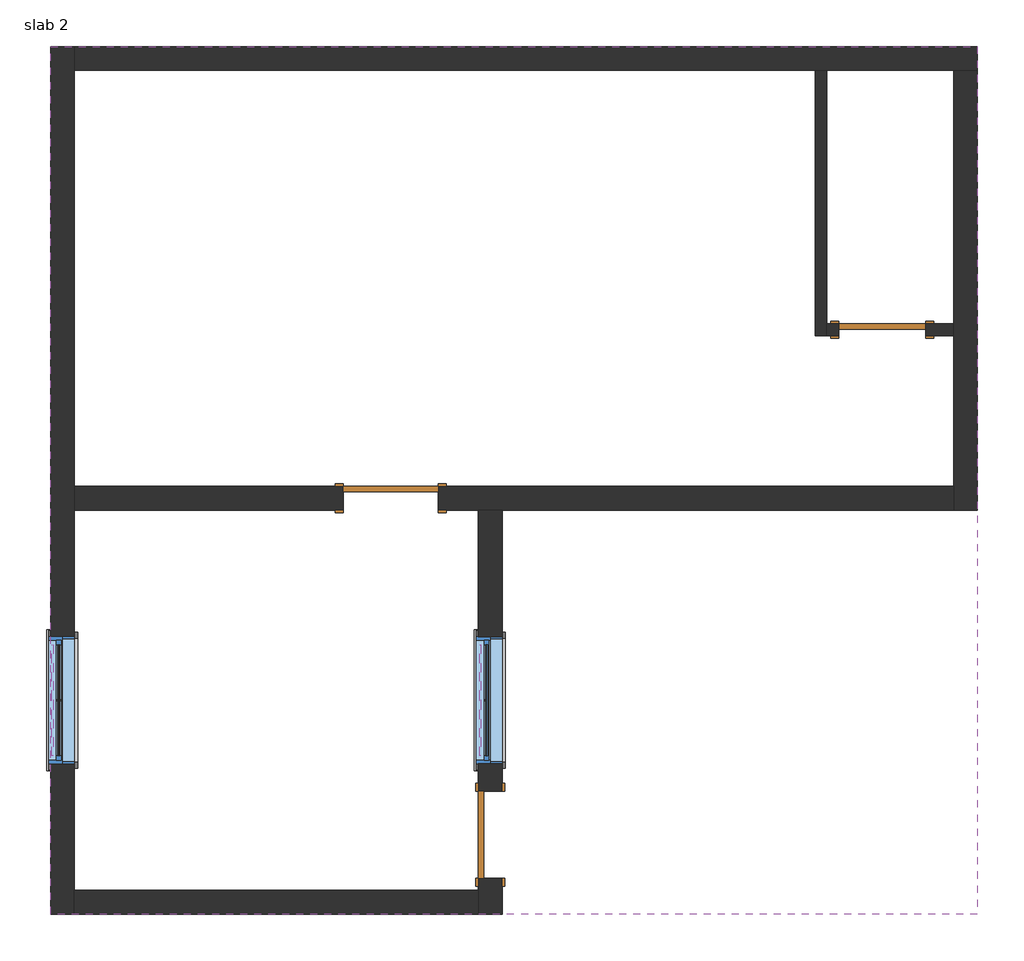
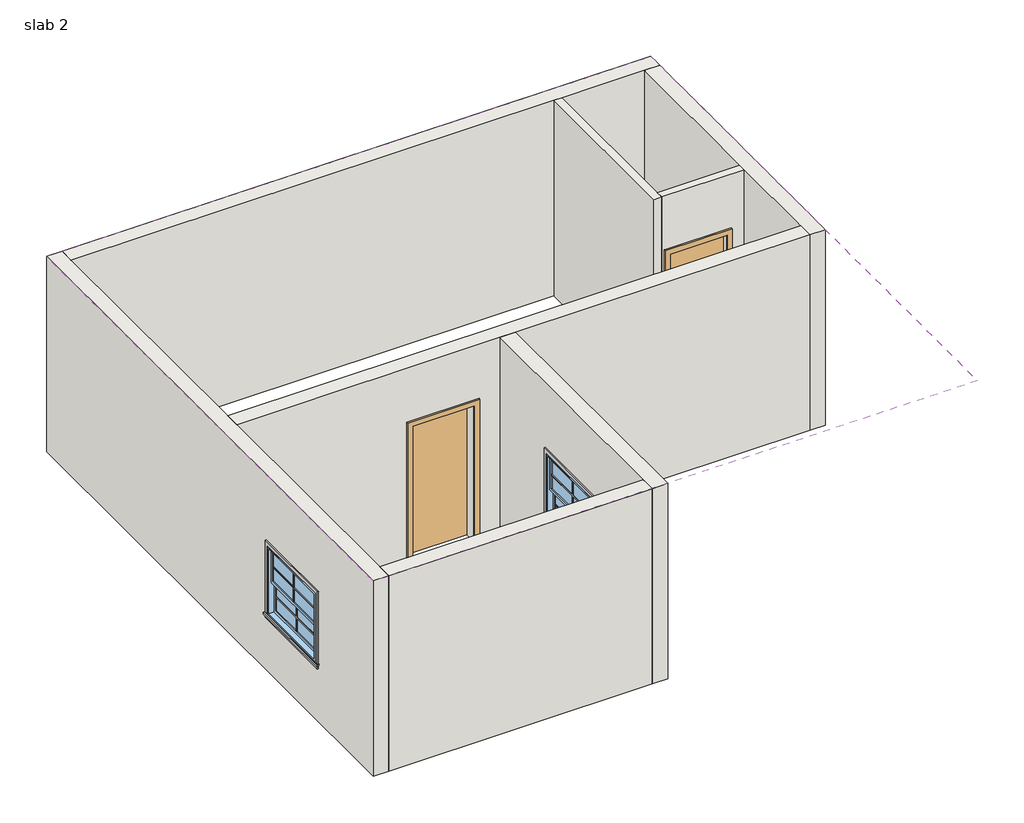
# One storey: 8 proxies, 8 walls, 3 doors, 2 windows, 1 roof.
"""IFC4 building model written with IfcOpenShell, lengths in millimetres."""

from ifc_helpers import new_model, si_unit, frame, origin, place, context, project, spatial, polyline, outline, extrude, faceted_brep, transform, mapped, element, save
from components import muntin_pattern_2x2_muntin_pattern_2x2_8b3f23e7, trim_window_exterior_flat_with_sill_f44f30ad, trim_window_interior_flat_picture_frame_1dce1945, single_flush_3_d_0ca8825f, single_flush_d2_19300210, single_flush_d2_53d9c022, window_double_hung_4_eadb0177

model = new_model("IFC4")

# Units and contexts
model_context = context("Model", 3, world=origin())
ifc_project = project(units=[si_unit("LENGTHUNIT", "METRE", prefix="MILLI")], contexts=[model_context])

# Site, building, storey
site = spatial("IfcSite", under=ifc_project)
building = spatial("IfcBuilding", under=site)
storey = spatial("IfcBuildingStorey", under=building, Name="slab 2", Elevation=6400.8)

# Proxies
placement = place(None, origin())
muntin_pattern_2x2_muntin_pattern_2x2_shape = muntin_pattern_2x2_muntin_pattern_2x2_8b3f23e7(model_context)
element("IfcBuildingElementProxy", 1, Name="Muntin Pattern_2x2 : Muntin Pattern_2x2", ObjectType="Muntin Pattern_2x2 : Muntin Pattern_2x2", at=placement, inside=storey, context=model_context, shape_type="MappedRepresentation", body=[
    mapped(muntin_pattern_2x2_muntin_pattern_2x2_shape, transform((-18769.9649593, 1832.2908097, 7870.825), x_axis=(0.0, 1.0, 0.0), y_axis=(-1.0, 0.0, 0.0), z_axis=(0.0, 0.0, 1.0))),
])
element("IfcBuildingElementProxy", 2, Name="Muntin Pattern_2x2 : Muntin Pattern_2x2", ObjectType="Muntin Pattern_2x2 : Muntin Pattern_2x2", at=placement, inside=storey, context=model_context, shape_type="MappedRepresentation", body=[
    mapped(muntin_pattern_2x2_muntin_pattern_2x2_shape, transform((-18725.5149593, 1832.2908097, 7391.4), x_axis=(0.0, 1.0, 0.0), y_axis=(-1.0, 0.0, 0.0), z_axis=(0.0, 0.0, 1.0))),
])
element("IfcBuildingElementProxy", 3, Name="Muntin Pattern_2x2 : Muntin Pattern_2x2", ObjectType="Muntin Pattern_2x2 : Muntin Pattern_2x2", at=placement, inside=storey, context=model_context, shape_type="MappedRepresentation", body=[
    mapped(muntin_pattern_2x2_muntin_pattern_2x2_shape, transform((-22884.7649593, 1832.2908097, 7870.825), x_axis=(0.0, 1.0, 0.0), y_axis=(-1.0, 0.0, 0.0), z_axis=(0.0, 0.0, 1.0))),
])
element("IfcBuildingElementProxy", 4, Name="Muntin Pattern_2x2 : Muntin Pattern_2x2", ObjectType="Muntin Pattern_2x2 : Muntin Pattern_2x2", at=placement, inside=storey, context=model_context, shape_type="MappedRepresentation", body=[
    mapped(muntin_pattern_2x2_muntin_pattern_2x2_shape, transform((-22840.3149593, 1832.2908097, 7391.4), x_axis=(0.0, 1.0, 0.0), y_axis=(-1.0, 0.0, 0.0), z_axis=(0.0, 0.0, 1.0))),
])
trim_window_exterior_flat_with_sill_shape = trim_window_exterior_flat_with_sill_f44f30ad(model_context)
element("IfcBuildingElementProxy", 5, Name="Trim-Window-Exterior-Flat : with Sill", ObjectType="Trim-Window-Exterior-Flat : with Sill", at=placement, inside=storey, context=model_context, shape_type="MappedRepresentation", body=[
    mapped(trim_window_exterior_flat_with_sill_shape, transform((-18804.8899593, 1832.2908097, 8382.0), x_axis=(0.0, -1.0, 0.0), y_axis=(0.0, 0.0, 1.0), z_axis=(-1.0, 0.0, 0.0))),
])
element("IfcBuildingElementProxy", 6, Name="Trim-Window-Exterior-Flat : with Sill", ObjectType="Trim-Window-Exterior-Flat : with Sill", at=placement, inside=storey, context=model_context, shape_type="MappedRepresentation", body=[
    mapped(trim_window_exterior_flat_with_sill_shape, transform((-22919.6899593, 1832.2908097, 8382.0), x_axis=(0.0, -1.0, 0.0), y_axis=(0.0, 0.0, 1.0), z_axis=(-1.0, 0.0, 0.0))),
])
trim_window_interior_flat_picture_frame_shape = trim_window_interior_flat_picture_frame_1dce1945(model_context)
element("IfcBuildingElementProxy", 7, Name="Trim-Window-Interior-Flat : Picture Frame", ObjectType="Trim-Window-Interior-Flat : Picture Frame", at=placement, inside=storey, context=model_context, shape_type="MappedRepresentation", body=[
    mapped(trim_window_interior_flat_picture_frame_shape, transform((-18576.2899593, 1832.2908097, 8382.0), x_axis=(0.0, 1.0, 0.0), y_axis=(0.0, 0.0, 1.0), z_axis=(1.0, 0.0, 0.0))),
])
element("IfcBuildingElementProxy", 8, Name="Trim-Window-Interior-Flat : Picture Frame", ObjectType="Trim-Window-Interior-Flat : Picture Frame", at=placement, inside=storey, context=model_context, shape_type="MappedRepresentation", body=[
    mapped(trim_window_interior_flat_picture_frame_shape, transform((-22691.0899593, 1832.2908097, 8382.0), x_axis=(0.0, 1.0, 0.0), y_axis=(0.0, 0.0, 1.0), z_axis=(1.0, 0.0, 0.0))),
])

# Doors
single_flush_3_d_shape = single_flush_3_d_0ca8825f(model_context)
element("IfcDoor", 9, ObjectType="Single-Flush : 3'd", at=placement, inside=storey, context=model_context, shape_type="MappedRepresentation", body=[
    mapped(single_flush_3_d_shape, transform((-19647.1461016, 3775.3908098, 6400.8), x_axis=(1.0, 0.0, 0.0), y_axis=(0.0, 1.0, 0.0), z_axis=(0.0, 0.0, 1.0))),
])
single_flush_d2_shape = single_flush_d2_19300210(model_context)
element("IfcDoor", 10, ObjectType="Single-Flush : d2", at=placement, inside=storey, context=model_context, shape_type="MappedRepresentation", body=[
    mapped(single_flush_d2_shape, transform((-14918.6899593, 5394.6408098, 6400.8), x_axis=(-1.0, 0.0, 0.0), y_axis=(0.0, -1.0, 0.0), z_axis=(0.0, 0.0, 1.0))),
])
single_flush_d2_2_shape = single_flush_d2_53d9c022(model_context)
element("IfcDoor", 11, ObjectType="Single-Flush : d2", at=placement, inside=storey, context=model_context, shape_type="MappedRepresentation", body=[
    mapped(single_flush_d2_2_shape, transform((-18690.5899593, 536.8908098, 6400.8), x_axis=(0.0, -1.0, 0.0), y_axis=(1.0, 0.0, 0.0), z_axis=(0.0, 0.0, 1.0))),
])

# Roof
element("IfcRoof", 12, ObjectType="6\" slab", at=placement, inside=storey, context=model_context, shape_type="SweptSolid", body=[
    extrude(outline(polyline([(-22919.6899593, 8118.7908098), (-14004.2899593, 8118.7908098), (-14004.2899593, -225.1091902), (-22919.6899593, -225.1091902), (-22919.6899593, 8118.7908098)])), frame((0.0, 0.0, 9448.8), z_axis=(0.0, 0.0, 1.0), x_axis=(1.0, 0.0, 0.0)), (0.0, 0.0, 1.0), 152.4),
])

# Walls
element("IfcWall", 13, ObjectType="4.5\" w 2", at=placement, inside=storey, context=model_context, shape_type="Brep", body=[
    faceted_brep([(-15566.3899593, 7890.1908098, 6400.8), (-15566.3899593, 5337.4908098, 6400.8), (-15566.3899593, 5337.4908098, 9448.8), (-15566.3899593, 7890.1908098, 9448.8), (-15452.0899593, 7890.1908098, 6400.8), (-15452.0899593, 7890.1908098, 9448.8), (-15452.0899593, 5451.7908098, 9448.8), (-15452.0899593, 5337.4908098, 9448.8), (-15452.0899593, 5337.4908098, 6400.8), (-15452.0899593, 5451.7908098, 6400.8)], [[[0, 1, 2, 3]], [[4, 5, 6, 7, 8, 9]], [[1, 0, 4, 9, 8]], [[3, 2, 7, 6, 5]], [[0, 3, 5, 4]], [[2, 1, 8, 7]]]),
])
element("IfcWall", 14, ObjectType="4.5\" w 2", at=placement, inside=storey, context=model_context, shape_type="SweptSolid", body=[
    extrude(outline(polyline([(6400.8, -15452.0899593), (6400.8, -15337.7899593), (8534.4, -15337.7899593), (8534.4, -14499.5899593), (6400.8, -14499.5899593), (6400.8, -14232.8899593), (9448.8, -14232.8899593), (9448.8, -15452.0899593), (6400.8, -15452.0899593)])), frame((0.0, 5337.4908098, 0.0), z_axis=(0.0, 1.0, 0.0), x_axis=(0.0, 0.0, 1.0)), (0.0, 0.0, 1.0), 114.3),
])
element("IfcWall", 15, ObjectType="9\" w 2", at=placement, inside=storey, context=model_context, shape_type="Brep", body=[
    faceted_brep([(-22691.0899593, -225.1091902, 6400.8), (-22691.0899593, 3.4908098, 6400.8), (-22691.0899593, 3661.0908098, 6400.8), (-22691.0899593, 3889.6908098, 6400.8), (-22691.0899593, 7890.1908098, 6400.8), (-22691.0899593, 8118.7908098, 6400.8), (-22691.0899593, 8118.7908098, 9448.8), (-22691.0899593, 7890.1908098, 9448.8), (-22691.0899593, 3889.6908098, 9448.8), (-22691.0899593, 3661.0908098, 9448.8), (-22691.0899593, 3.4908098, 9448.8), (-22691.0899593, -225.1091902, 9448.8), (-22691.0899593, 1222.6908097, 8382.0), (-22691.0899593, 2441.8908097, 8382.0), (-22691.0899593, 2441.8908097, 7315.2), (-22691.0899593, 1222.6908097, 7315.2), (-22919.6899593, -225.1091902, 6400.8), (-22919.6899593, -225.1091902, 9448.8), (-22919.6899593, 8118.7908098, 9448.8), (-22919.6899593, 8118.7908098, 6400.8), (-22919.6899593, 1222.6908097, 8382.0), (-22919.6899593, 1222.6908097, 7315.2), (-22919.6899593, 2441.8908097, 7315.2), (-22919.6899593, 2441.8908097, 8382.0)], [[[0, 1, 2, 3, 4, 5, 6, 7, 8, 9, 10, 11], [12, 13, 14, 15]], [[16, 17, 18, 19], [20, 21, 22, 23]], [[5, 4, 3, 2, 1, 0, 16, 19]], [[11, 10, 9, 8, 7, 6, 18, 17]], [[6, 5, 19, 18]], [[0, 11, 17, 16]], [[21, 20, 12, 15]], [[22, 21, 15, 14]], [[23, 22, 14, 13]], [[20, 23, 13, 12]]]),
])
element("IfcWall", 16, ObjectType="9\" w 2", at=placement, inside=storey, context=model_context, shape_type="Brep", body=[
    faceted_brep([(-22691.0899593, 7890.1908098, 6400.8), (-15566.3899593, 7890.1908098, 6400.8), (-15452.0899593, 7890.1908098, 6400.8), (-14232.8899593, 7890.1908098, 6400.8), (-14004.2899593, 7890.1908098, 6400.8), (-14004.2899593, 7890.1908098, 9448.8), (-14232.8899593, 7890.1908098, 9448.8), (-15452.0899593, 7890.1908098, 9448.8), (-15566.3899593, 7890.1908098, 9448.8), (-22691.0899593, 7890.1908098, 9448.8), (-22691.0899593, 8118.7908098, 6400.8), (-22691.0899593, 8118.7908098, 9448.8), (-14004.2899593, 8118.7908098, 9448.8), (-14004.2899593, 8118.7908098, 6400.8)], [[[0, 1, 2, 3, 4, 5, 6, 7, 8, 9]], [[10, 11, 12, 13]], [[4, 3, 2, 1, 0, 10, 13]], [[9, 8, 7, 6, 5, 12, 11]], [[0, 9, 11, 10]], [[5, 4, 13, 12]]]),
])
element("IfcWall", 17, ObjectType="9\" w 2", at=placement, inside=storey, context=model_context, shape_type="Brep", body=[
    faceted_brep([(-14232.8899593, 7890.1908098, 6400.8), (-14232.8899593, 5451.7908098, 6400.8), (-14232.8899593, 5337.4908098, 6400.8), (-14232.8899593, 3889.6908098, 6400.8), (-14232.8899593, 3661.0908098, 6400.8), (-14232.8899593, 3661.0908098, 9448.8), (-14232.8899593, 3889.6908098, 9448.8), (-14232.8899593, 5337.4908098, 9448.8), (-14232.8899593, 5451.7908098, 9448.8), (-14232.8899593, 7890.1908098, 9448.8), (-14004.2899593, 7890.1908098, 6400.8), (-14004.2899593, 7890.1908098, 9448.8), (-14004.2899593, 3661.0908098, 9448.8), (-14004.2899593, 3661.0908098, 6400.8)], [[[0, 1, 2, 3, 4, 5, 6, 7, 8, 9]], [[10, 11, 12, 13]], [[4, 3, 2, 1, 0, 10, 13]], [[9, 8, 7, 6, 5, 12, 11]], [[0, 9, 11, 10]], [[5, 4, 13, 12]]]),
])
element("IfcWall", 18, ObjectType="9\" w 2", at=placement, inside=storey, context=model_context, shape_type="Brep", body=[
    faceted_brep([(-14232.8899593, 3889.6908098, 6400.8), (-19189.9461016, 3889.6908098, 6400.8), (-19189.9461016, 3889.6908098, 8534.4), (-20104.3461016, 3889.6908098, 8534.4), (-20104.3461016, 3889.6908098, 6400.8), (-22691.0899593, 3889.6908098, 6400.8), (-22691.0899593, 3889.6908098, 9448.8), (-14232.8899593, 3889.6908098, 9448.8), (-19189.9461016, 3661.0908098, 8534.4), (-19189.9461016, 3661.0908098, 6400.8), (-18804.8899593, 3661.0908098, 6400.8), (-18576.2899593, 3661.0908098, 6400.8), (-14232.8899593, 3661.0908098, 6400.8), (-14232.8899593, 3661.0908098, 9448.8), (-18576.2899593, 3661.0908098, 9448.8), (-18804.8899593, 3661.0908098, 9448.8), (-22691.0899593, 3661.0908098, 9448.8), (-22691.0899593, 3661.0908098, 6400.8), (-20104.3461016, 3661.0908098, 6400.8), (-20104.3461016, 3661.0908098, 8534.4)], [[[0, 1, 2, 3, 4, 5, 6, 7]], [[8, 9, 10, 11, 12, 13, 14, 15, 16, 17, 18, 19]], [[18, 17, 5, 4]], [[12, 11, 10, 9, 1, 0]], [[7, 6, 16, 15, 14, 13]], [[0, 7, 13, 12]], [[6, 5, 17, 16]], [[2, 1, 9, 8]], [[3, 2, 8, 19]], [[4, 3, 19, 18]]]),
])
element("IfcWall", 19, ObjectType="9\" w 2", at=placement, inside=storey, context=model_context, shape_type="Brep", body=[
    faceted_brep([(-18804.8899593, 117.7908098, 8534.4), (-18804.8899593, 117.7908098, 6400.8), (-18804.8899593, 3.4908098, 6400.8), (-18804.8899593, -225.1091902, 6400.8), (-18804.8899593, -225.1091902, 9448.8), (-18804.8899593, 3.4908098, 9448.8), (-18804.8899593, 3661.0908098, 9448.8), (-18804.8899593, 3661.0908098, 6400.8), (-18804.8899593, 955.9908098, 6400.8), (-18804.8899593, 955.9908098, 8534.4), (-18804.8899593, 1222.6908097, 8382.0), (-18804.8899593, 1222.6908097, 7315.2), (-18804.8899593, 2441.8908097, 7315.2), (-18804.8899593, 2441.8908097, 8382.0), (-18576.2899593, -225.1091902, 6400.8), (-18576.2899593, 117.7908098, 6400.8), (-18576.2899593, 117.7908098, 8534.4), (-18576.2899593, 955.9908098, 8534.4), (-18576.2899593, 955.9908098, 6400.8), (-18576.2899593, 3661.0908098, 6400.8), (-18576.2899593, 3661.0908098, 9448.8), (-18576.2899593, -225.1091902, 9448.8), (-18576.2899593, 1222.6908097, 8382.0), (-18576.2899593, 2441.8908097, 8382.0), (-18576.2899593, 2441.8908097, 7315.2), (-18576.2899593, 1222.6908097, 7315.2)], [[[0, 1, 2, 3, 4, 5, 6, 7, 8, 9], [10, 11, 12, 13]], [[14, 15, 16, 17, 18, 19, 20, 21], [22, 23, 24, 25]], [[8, 7, 19, 18]], [[3, 2, 1, 15, 14]], [[6, 5, 4, 21, 20]], [[7, 6, 20, 19]], [[4, 3, 14, 21]], [[16, 15, 1, 0]], [[17, 16, 0, 9]], [[18, 17, 9, 8]], [[11, 10, 22, 25]], [[12, 11, 25, 24]], [[13, 12, 24, 23]], [[10, 13, 23, 22]]]),
])
element("IfcWall", 20, ObjectType="9\" w 2", at=placement, inside=storey, context=model_context, shape_type="SweptSolid", body=[
    extrude(outline(polyline([(-22691.0899593, 3.4908098), (-18804.8899593, 3.4908098), (-18804.8899593, -225.1091902), (-22691.0899593, -225.1091902), (-22691.0899593, 3.4908098)])), frame((0.0, 0.0, 6400.8), z_axis=(0.0, 0.0, 1.0), x_axis=(1.0, 0.0, 0.0)), (0.0, 0.0, 1.0), 3048.0),
])

# Windows
window_double_hung_4_shape = window_double_hung_4_eadb0177(model_context)
element("IfcWindow", 21, ObjectType="Window-Double-Hung : 4'", at=placement, inside=storey, context=model_context, shape_type="MappedRepresentation", body=[
    mapped(window_double_hung_4_shape, transform((-18690.5899593, 1832.2908097, 6400.8), x_axis=(0.0, 1.0, 0.0), y_axis=(-1.0, 0.0, 0.0), z_axis=(0.0, 0.0, 1.0))),
])
element("IfcWindow", 22, ObjectType="Window-Double-Hung : 4'", at=placement, inside=storey, context=model_context, shape_type="MappedRepresentation", body=[
    mapped(window_double_hung_4_shape, transform((-22805.3899593, 1832.2908097, 6400.8), x_axis=(0.0, 1.0, 0.0), y_axis=(-1.0, 0.0, 0.0), z_axis=(0.0, 0.0, 1.0))),
])

save(model, "model.ifc")

# Revit data of these elements
# Type "Muntin Pattern_2x2 : Muntin Pattern_2x2"
#   Width [instance default] = 4' - 0"
#   Thickness = 0' - 0 1/2"
#   Height [instance default] = 4' - 0"
#   Distance = 0' - 0 3/4"
#   Interior Material [instance default] = none
#   Exterior Material [instance default] = none
#   Default Elevation = 0
# Type "Trim-Window-Exterior-Flat : with Sill"
#   Trim Width = 0' - 2 1/4"
#   Trim Thickness_Picture Frame = 0' - 1 1/4"
#   Trim Thickness_with Sill = 0' - 0 3/4"
#   Sill Thickness = 0' - 1 1/4"
#   Opening Width [instance default] = 2' - 0"
#   Opening Height [instance default] = 3' - 0"
#   Default Elevation = 4' - 0"
#   Sill = yes
#   Picture Frame = no
#   Trim Material [instance default] = none
# Type "Trim-Window-Interior-Flat : Picture Frame"
#   Trim Thickness_Picture Frame = 0' - 1 1/4"
#   Trim Width = 0' - 2 1/4"
#   Trim Thickness_with Sill = 0' - 0 3/4"
#   Sill Thickness = 0' - 1 1/4"
#   Opening Width [instance default] = 2' - 0"
#   Opening Height [instance default] = 3' - 0"
#   Default Elevation = 4' - 0"
#   Sill = no
#   Picture Frame = yes
#   Trim Material [instance default] = none
# Type "Single-Flush : 3'd"
#   Type Mark = "13"
#   Construction Type Id = "MDOOR"
#   Assembly Code = "C1020"
#   Analytic Construction = "Metal"
#   Thickness = 0' - 2"
#   Heat Transfer Coefficient (U) = 0.651978 BTU/(h·ft²·°F)
#   Height = 7' - 0"
#   Trim Projection Ext = 0' - 1"
#   Trim Projection Int = 0' - 1"
#   Trim Width = 0' - 3"
#   Width = 3' - 0"
#   Define Thermal Properties by = 1
#   Door Material = Door - Panel
#   Frame Material = Door - Frame
#   Visual Light Transmittance = 0
#   Solar Heat Gain Coefficient = 0
#   Function = (empty or 0)
#   Wall Closure = (empty or 0)
# Type "Single-Flush : d2"
#   Type Mark = "9"
#   Construction Type Id = "MDOOR"
#   Assembly Code = "C1020"
#   Analytic Construction = "Metal"
#   Thickness = 0' - 2"
#   Heat Transfer Coefficient (U) = 0.651978 BTU/(h·ft²·°F)
#   Height = 7' - 0"
#   Trim Projection Ext = 0' - 1"
#   Trim Projection Int = 0' - 1"
#   Trim Width = 0' - 3"
#   Width = 2' - 9"
#   Define Thermal Properties by = 1
#   Door Material = Door - Panel
#   Frame Material = Door - Frame
#   Visual Light Transmittance = 0
#   Solar Heat Gain Coefficient = 0
#   Function = (empty or 0)
#   Wall Closure = (empty or 0)
# Type "6\" slab"
#   Assembly Code = "B1020"
#   Layers, outside or top first: 0' - 6" no material (function 1)
# Type "4.5\" w 2"
#   Assembly Code = "B2010"
#   Layers, outside or top first: 0' - 4 1/2" no material (function 1)
# Type "9\" w 2"
#   Assembly Code = "B2010"
#   Layers, outside or top first: 0' - 9" no material (function 1)
# Type "Window-Double-Hung : 4'"
#   Type Mark = "24"
#   Fire Rating = "0.5h"
#   Construction Type Id = "DG-DR"
#   Assembly Code = "B2020100"
#   Analytic Construction = "Double glazing - domestic"
#   Wall Thickness [instance default] = 0' - 6"
#   Window Inset [instance default] = 0' - 0"
#   Visual Light Transmittance = 0.81
#   Thermal Resistance (R) = 1.8146 (h·ft²·°F)/BTU
#   Solar Heat Gain Coefficient = 0.76
#   Muntin Width = 3' - 6"
#   Muntin Height = 1' - 5 1/8"
#   Interior Wall Closure [instance default] = 0' - 1 1/2"
#   Rough Width = 4' - 0 1/2"
#   Rough Height = 3' - 6 1/2"
#   Frame Extension [instance default] = 0' - 1 1/4"
#   Exterior Wall Closure [instance default] = 0' - 0 1/2"
#   Extension Jamb [instance default] = 0' - 1 1/2"
#   Heat Transfer Coefficient (U) = 0.5511 BTU/(h·ft²·°F)
#   Height = 3' - 6"
#   Width = 4' - 0"
#   Top Muntin Visibility = yes
#   Indicator Visibility [instance default] = yes
#   Extension Jamb Visibility [instance default] = yes
#   Interior Trim Visibility [instance default] = yes
#   Exterior Trim Visibility [instance default] = yes
#   Define Thermal Properties by = 1
#   Bottom Muntin Visibility = yes
#   Muntin Pattern = Muntin Pattern_2x2 : Muntin Pattern_2x2
#   Interior Trim Material = Wood - Stained
#   Interior Trim = Trim-Window-Interior-Flat : Picture Frame
#   Exterior Trim Material = Clad - White
#   Exterior Trim = Trim-Window-Exterior-Flat : with Sill
#   Glass Panel Material = Glass
#   Exterior Frame Material = Clad - White
#   Interior Frame Material = Wood - Stained
#   Wall Closure = (empty or 0)
# Elements 1, 2, 3, 4 (IfcBuildingElementProxy, "Muntin Pattern_2x2 : Muntin Pattern_2x2")
#   Width = 3' - 6"
#   Height = 1' - 5 1/8"
#   Interior Material = Wood - Stained
#   Exterior Material = Clad - White
#   Phase Created = New Construction
#   Materials on its faces: "Clad - White", "Wood - Stained"
# Elements 5, 6 (IfcBuildingElementProxy, "Trim-Window-Exterior-Flat : with Sill")
#   Opening Width = 4' - 0"
#   Opening Height = 3' - 6"
#   Trim Material = Clad - White
#   Phase Created = New Construction
#   Materials on its faces: "Clad - White"
# Elements 7, 8 (IfcBuildingElementProxy, "Trim-Window-Interior-Flat : Picture Frame")
#   Opening Width = 4' - 0"
#   Opening Height = 3' - 6"
#   Trim Material = Wood - Stained
#   Phase Created = New Construction
#   Materials on its faces: "Wood - Stained"
# Element 9 (IfcDoor, "Single-Flush : 3'd")
#   Phase Created = New Construction
#   Materials on its faces: "Door - Frame", "Door - Panel"
# Elements 10, 11 (IfcDoor, "Single-Flush : d2")
#   Phase Created = New Construction
#   Materials on its faces: "Door - Frame", "Door - Panel"
# Element 12 (IfcRoof, "6\" slab")
#   built-in parameter 1001705 = 31.5 (stored number, unit not read)
#   built-in parameter 1001701 = 10 (stored number, unit not read)
#   built-in parameter 1001710 = 33615
#   Phase Created = New Construction
#   Materials on its faces: "Default Roof"
# Elements 13, 14 (IfcWall, "4.5\" w 2")
#   Top Offset = 0' - 0"
#   Base Offset = 0' - 0"
#   Unconnected Height = 10' - 0"
#   wall height = 10' - 0"
#   Phase Created = New Construction
#   Base Constraint = slab 2
#   Materials on its faces: "Default Wall"
# Elements 15, 16, 17, 18, 19, 20 (IfcWall, "9\" w 2")
#   Top Offset = 0' - 0"
#   Base Offset = 0' - 0"
#   Unconnected Height = 10' - 0"
#   wall height = 10' - 0"
#   Phase Created = New Construction
#   Base Constraint = slab 2
#   Materials on its faces: "Default Wall"
# Element 21 (IfcWindow, "Window-Double-Hung : 4'")
#   Mark = "18"
#   Window Inset = 0' - 0"
#   Interior Wall Closure = 0' - 1 1/2"
#   Frame Extension = 0' - 1 1/4"
#   Exterior Wall Closure = 0' - 0 1/2"
#   Interior Trim Visibility = yes
#   Indicator Visibility = yes
#   Exterior Trim Visibility = yes
#   Phase Created = New Construction
#   Materials on its faces: "Wood - Stained", "Glass", "Clad - White"
# Element 22 (IfcWindow, "Window-Double-Hung : 4'")
#   Mark = "19"
#   Window Inset = 0' - 0"
#   Interior Wall Closure = 0' - 1 1/2"
#   Frame Extension = 0' - 1 1/4"
#   Exterior Wall Closure = 0' - 0 1/2"
#   Interior Trim Visibility = yes
#   Indicator Visibility = yes
#   Exterior Trim Visibility = yes
#   Phase Created = New Construction
#   Materials on its faces: "Wood - Stained", "Glass", "Clad - White"
# Materials
#   "Door - Panel": class "Wood", colour RGB 210 159 95, transparency 0, Cost = 0
#   "Door - Frame": colour RGB 118 70 51, transparency 0, Cost = 0
#   "Wood - Stained": class "Wood", colour RGB 224 178 126, transparency 0, Cost = 0
#   "Clad - White": class "Wood", colour RGB 242 242 238, transparency 0, Cost = 0
#   "Glass": class "Glass", colour RGB 0 128 192, transparency 0.75, Description = "Soda Lime Glass", Cost = 0
#   "Default Roof": colour RGB 88 101 114, transparency 0, Cost = 0
#   "Default Wall": colour RGB 128 128 128, transparency 0, Cost = 0
